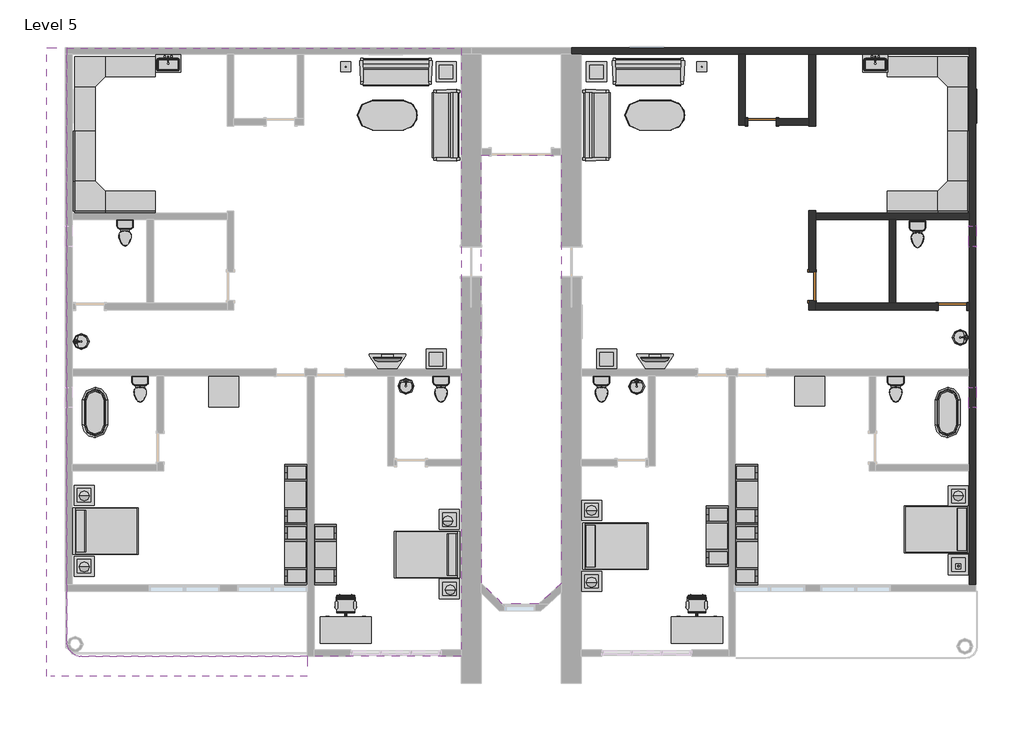
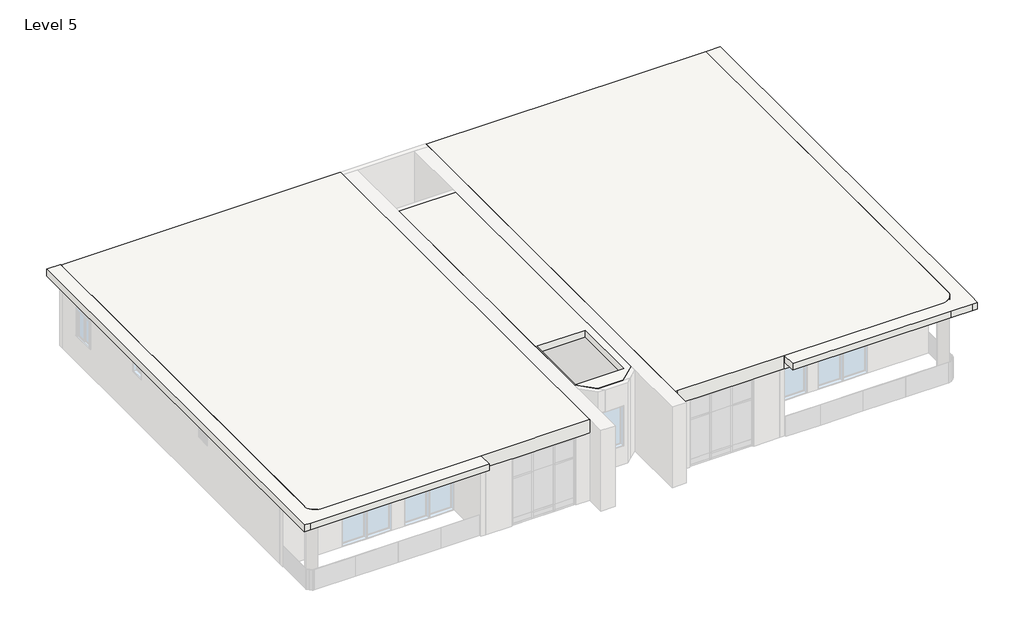
# One storey, part 3 of 3: 42 furniture elements, 14 flow terminals, 10 light fixtures, 9 walls, 3 doors, 3 slabs, 3 windows.
"""IFC4 building model written with IfcOpenShell, lengths in millimetres."""

from ifc_helpers import new_model, si_unit, point, frame, frame_2d, origin, place, context, project, spatial, polyline, circle_curve, trimmed, segment, composite_curve, outline, extrude, faceted_brep, transform, mapped, element, save
from components import door_2703ae13, door_10fd3a06, flow_terminal_38af2918, flow_terminal_d49f872f, toilet_domestic_3d_toilet_domestic_3d_f7549cf7, toilet_domestic_3d_toilet_domestic_3d_183bbd19, flow_terminal_b374fae2, furniture_07436f11, furniture_096e7f55, chair_task_arms_chair_task_arms_fa5a08ef, furniture_072f6425, furniture_cf0b6580, furniture_aff9b2fb, furniture_56245f3a, tv_stand_tv_stand_6ce107e5, furniture_b5c51a22, furniture_2c34a4f9, furniture_4d44e21c, furniture_45e3acac, light_fixture_100w_120v_8564026f, table_lamp_hemispheric_60w_120v_02721d88, window_0038ecf3, window_54100e87

model = new_model("IFC4")

# Units and contexts
model_context = context("Model", 3, world=origin())
ifc_project = project(units=[si_unit("LENGTHUNIT", "METRE", prefix="MILLI")], contexts=[model_context])

# Site, building, storey
site = spatial("IfcSite", under=ifc_project)
building = spatial("IfcBuilding", under=site)
storey = spatial("IfcBuildingStorey", under=building, Name="Level 5", Elevation=14630.4)

# Doors
placement = place(None, origin())
door_shape = door_2703ae13(model_context)
element("IfcDoor", 1, ObjectType="Door-Single-Panel.0001 : 34\" x 80\"", at=placement, inside=storey, context=model_context, shape_type="MappedRepresentation", body=[
    mapped(door_shape, transform((2522.0012296, 9464.0758558, 14630.4), x_axis=(-1.0, 0.0, 0.0), y_axis=(0.0, -1.0, 0.0), z_axis=(0.0, 0.0, 1.0))),
])
door_2_shape = door_10fd3a06(model_context)
element("IfcDoor", 2, ObjectType="Door-Single-Panel.0001 : 34\" x 80\"", at=placement, inside=storey, context=model_context, shape_type="MappedRepresentation", body=[
    mapped(door_2_shape, transform((8313.2012296, 3850.6758558, 14630.4), x_axis=(1.0, 0.0, 0.0), y_axis=(0.0, 1.0, 0.0), z_axis=(0.0, 0.0, 1.0))),
])
element("IfcDoor", 3, ObjectType="Door-Single-Panel.0001 : 34\" x 80\"", at=placement, inside=storey, context=model_context, shape_type="MappedRepresentation", body=[
    mapped(door_2_shape, transform((4046.0012296, 4460.2758558, 14630.4), x_axis=(0.0, -1.0, 0.0), y_axis=(1.0, 0.0, 0.0), z_axis=(0.0, 0.0, 1.0))),
])

# Flow terminals
flow_terminal_shape = flow_terminal_38af2918(model_context)
element("IfcFlowTerminal", 4, ObjectType="Sink Kitchen-Single : 30\" x 21\"", at=placement, inside=storey, context=model_context, shape_type="MappedRepresentation", body=[
    mapped(flow_terminal_shape, transform((-15540.388011, 11239.7304546, 14630.4), x_axis=(1.0, 0.0, 0.0), y_axis=(0.0, 1.0, 0.0), z_axis=(0.0, 0.0, 1.0))),
])
element("IfcFlowTerminal", 5, ObjectType="Sink Kitchen-Single : 30\" x 21\"", at=placement, inside=storey, context=model_context, shape_type="MappedRepresentation", body=[
    mapped(flow_terminal_shape, transform((5948.011989, 11239.7304546, 14630.4), x_axis=(1.0, 0.0, 0.0), y_axis=(0.0, 1.0, 0.0), z_axis=(0.0, 0.0, 1.0))),
])
flow_terminal_2_shape = flow_terminal_d49f872f(model_context)
element("IfcFlowTerminal", 6, ObjectType="Sink Vanity-Round : 19\" x 19\"", at=placement, inside=storey, context=model_context, shape_type="MappedRepresentation", body=[
    mapped(flow_terminal_2_shape, transform((-18084.6070794, 2687.2241152, 14630.4), x_axis=(0.0, 1.0, 0.0), y_axis=(-1.0, 0.0, 0.0), z_axis=(0.0, 0.0, 1.0))),
])
element("IfcFlowTerminal", 7, ObjectType="Sink Vanity-Round : 19\" x 19\"", at=placement, inside=storey, context=model_context, shape_type="MappedRepresentation", body=[
    mapped(flow_terminal_2_shape, transform((8462.2249463, 3007.5275963, 14630.4), x_axis=(0.0, -1.0, 0.0), y_axis=(1.0, 0.0, 0.0), z_axis=(0.0, 0.0, 1.0))),
])
element("IfcFlowTerminal", 8, ObjectType="Sink Vanity-Round : 19\" x 19\"", at=placement, inside=storey, context=model_context, shape_type="MappedRepresentation", body=[
    mapped(flow_terminal_2_shape, transform((-8395.050511, 1341.8921141, 14630.4), x_axis=(1.0, 0.0, 0.0), y_axis=(0.0, 1.0, 0.0), z_axis=(0.0, 0.0, 1.0))),
])
element("IfcFlowTerminal", 9, ObjectType="Sink Vanity-Round : 19\" x 19\"", at=placement, inside=storey, context=model_context, shape_type="MappedRepresentation", body=[
    mapped(flow_terminal_2_shape, transform((-1384.650511, 1331.0855344, 14630.4), x_axis=(1.0, 0.0, 0.0), y_axis=(0.0, 1.0, 0.0), z_axis=(0.0, 0.0, 1.0))),
])
toilet_domestic_3d_toilet_domestic_3d_shape = toilet_domestic_3d_toilet_domestic_3d_f7549cf7(model_context)
toilet_domestic_3d_toilet_domestic_3d_2_shape = toilet_domestic_3d_toilet_domestic_3d_183bbd19(model_context)
element("IfcFlowTerminal", 10, ObjectType="Toilet-Domestic-3D : Toilet-Domestic-3D", at=placement, inside=storey, context=model_context, shape_type="MappedRepresentation", body=[
    mapped(toilet_domestic_3d_toilet_domestic_3d_shape, transform((6586.0012296, 1247.7798284, 14630.4), x_axis=(1.0, 0.0, 0.0), y_axis=(0.0, 1.0, 0.0), z_axis=(0.0, 0.0, 1.0))),
    mapped(toilet_domestic_3d_toilet_domestic_3d_2_shape, transform((6586.0012296, 1247.7798284, 14630.4), x_axis=(1.0, 0.0, 0.0), y_axis=(0.0, 1.0, 0.0), z_axis=(0.0, 0.0, 1.0))),
])
element("IfcFlowTerminal", 11, ObjectType="Toilet-Domestic-3D : Toilet-Domestic-3D", at=placement, inside=storey, context=model_context, shape_type="MappedRepresentation", body=[
    mapped(toilet_domestic_3d_toilet_domestic_3d_shape, transform((-2354.7987704, 1247.7798284, 14630.4), x_axis=(1.0, 0.0, 0.0), y_axis=(0.0, 1.0, 0.0), z_axis=(0.0, 0.0, 1.0))),
    mapped(toilet_domestic_3d_toilet_domestic_3d_2_shape, transform((-2354.7987704, 1247.7798284, 14630.4), x_axis=(1.0, 0.0, 0.0), y_axis=(0.0, 1.0, 0.0), z_axis=(0.0, 0.0, 1.0))),
])
element("IfcFlowTerminal", 12, ObjectType="Toilet-Domestic-3D : Toilet-Domestic-3D", at=placement, inside=storey, context=model_context, shape_type="MappedRepresentation", body=[
    mapped(toilet_domestic_3d_toilet_domestic_3d_shape, transform((-16375.5987704, 1247.7798284, 14630.4), x_axis=(1.0, 0.0, 0.0), y_axis=(0.0, 1.0, 0.0), z_axis=(0.0, 0.0, 1.0))),
    mapped(toilet_domestic_3d_toilet_domestic_3d_2_shape, transform((-16375.5987704, 1247.7798284, 14630.4), x_axis=(1.0, 0.0, 0.0), y_axis=(0.0, 1.0, 0.0), z_axis=(0.0, 0.0, 1.0))),
])
element("IfcFlowTerminal", 13, ObjectType="Toilet-Domestic-3D : Toilet-Domestic-3D", at=placement, inside=storey, context=model_context, shape_type="MappedRepresentation", body=[
    mapped(toilet_domestic_3d_toilet_domestic_3d_shape, transform((-16832.7987704, 5997.5798284, 14630.4), x_axis=(1.0, 0.0, 0.0), y_axis=(0.0, 1.0, 0.0), z_axis=(0.0, 0.0, 1.0))),
    mapped(toilet_domestic_3d_toilet_domestic_3d_2_shape, transform((-16832.7987704, 5997.5798284, 14630.4), x_axis=(1.0, 0.0, 0.0), y_axis=(0.0, 1.0, 0.0), z_axis=(0.0, 0.0, 1.0))),
])
element("IfcFlowTerminal", 14, ObjectType="Toilet-Domestic-3D : Toilet-Domestic-3D", at=placement, inside=storey, context=model_context, shape_type="MappedRepresentation", body=[
    mapped(toilet_domestic_3d_toilet_domestic_3d_shape, transform((7246.4012296, 5946.7798284, 14630.4), x_axis=(1.0, 0.0, 0.0), y_axis=(0.0, 1.0, 0.0), z_axis=(0.0, 0.0, 1.0))),
    mapped(toilet_domestic_3d_toilet_domestic_3d_2_shape, transform((7246.4012296, 5946.7798284, 14630.4), x_axis=(1.0, 0.0, 0.0), y_axis=(0.0, 1.0, 0.0), z_axis=(0.0, 0.0, 1.0))),
])
element("IfcFlowTerminal", 15, ObjectType="Toilet-Domestic-3D : Toilet-Domestic-3D", at=placement, inside=storey, context=model_context, shape_type="MappedRepresentation", body=[
    mapped(toilet_domestic_3d_toilet_domestic_3d_shape, transform((-7231.5987704, 1247.7798284, 14630.4), x_axis=(1.0, 0.0, 0.0), y_axis=(0.0, 1.0, 0.0), z_axis=(0.0, 0.0, 1.0))),
    mapped(toilet_domestic_3d_toilet_domestic_3d_2_shape, transform((-7231.5987704, 1247.7798284, 14630.4), x_axis=(1.0, 0.0, 0.0), y_axis=(0.0, 1.0, 0.0), z_axis=(0.0, 0.0, 1.0))),
])
flow_terminal_3_shape = flow_terminal_b374fae2(model_context)
element("IfcFlowTerminal", 16, ObjectType="Tub-Free Standing-3D : 30\" x 60\"", at=placement, inside=storey, context=model_context, shape_type="MappedRepresentation", body=[
    mapped(flow_terminal_3_shape, transform((-17747.1987704, 624.8758558, 14630.4), x_axis=(1.0, 0.0, 0.0), y_axis=(0.0, 1.0, 0.0), z_axis=(0.0, 0.0, 1.0))),
])
element("IfcFlowTerminal", 17, ObjectType="Tub-Free Standing-3D : 30\" x 60\"", at=placement, inside=storey, context=model_context, shape_type="MappedRepresentation", body=[
    mapped(flow_terminal_3_shape, transform((8160.8012296, 624.8758558, 14630.4), x_axis=(1.0, 0.0, 0.0), y_axis=(0.0, 1.0, 0.0), z_axis=(0.0, 0.0, 1.0))),
])

# Furniture
furniture_shape = furniture_07436f11(model_context)
element("IfcFurniture", 18, ObjectType="96\" x 96\"", at=placement, inside=storey, context=model_context, shape_type="MappedRepresentation", body=[
    mapped(furniture_shape, transform((-18275.8670182, 11991.0988634, 14630.4), x_axis=(1.0, 0.0, 0.0), y_axis=(0.0, 1.0, 0.0), z_axis=(0.0, 0.0, 1.0))),
])
element("IfcFurniture", 19, ObjectType="96\" x 96\"", at=placement, inside=storey, context=model_context, shape_type="MappedRepresentation", body=[
    mapped(furniture_shape, transform((9316.2242372, 11364.3441035, 14630.4), x_axis=(0.0, -1.0, 0.0), y_axis=(1.0, 0.0, 0.0), z_axis=(0.0, 0.0, 1.0))),
])
furniture_2_shape = furniture_096e7f55(model_context)
element("IfcFurniture", 20, ObjectType="Bed-Shaker : Double 56\" x 78\"", at=placement, inside=storey, context=model_context, shape_type="MappedRepresentation", body=[
    mapped(furniture_2_shape, transform((-18407.5987704, -2962.8741442, 14630.4), x_axis=(0.0, 1.0, 0.0), y_axis=(-1.0, 0.0, 0.0), z_axis=(0.0, 0.0, 1.0))),
])
element("IfcFurniture", 21, ObjectType="Bed-Shaker : Double 56\" x 78\"", at=placement, inside=storey, context=model_context, shape_type="MappedRepresentation", body=[
    mapped(furniture_2_shape, transform((-6672.7987704, -3712.1741442, 14630.4), x_axis=(0.0, -1.0, 0.0), y_axis=(1.0, 0.0, 0.0), z_axis=(0.0, 0.0, 1.0))),
])
element("IfcFurniture", 22, ObjectType="Bed-Shaker : Double 56\" x 78\"", at=placement, inside=storey, context=model_context, shape_type="MappedRepresentation", body=[
    mapped(furniture_2_shape, transform((-2913.5987704, -3420.0741442, 14630.4), x_axis=(0.0, 1.0, 0.0), y_axis=(-1.0, 0.0, 0.0), z_axis=(0.0, 0.0, 1.0))),
])
element("IfcFurniture", 23, ObjectType="Bed-Shaker : Double 56\" x 78\"", at=placement, inside=storey, context=model_context, shape_type="MappedRepresentation", body=[
    mapped(furniture_2_shape, transform((8821.2012296, -2950.1741442, 14630.4), x_axis=(0.0, -1.0, 0.0), y_axis=(1.0, 0.0, 0.0), z_axis=(0.0, 0.0, 1.0))),
])
chair_task_arms_chair_task_arms_shape = chair_task_arms_chair_task_arms_fa5a08ef(model_context)
element("IfcFurniture", 24, ObjectType="Chair-Task Arms : Chair-Task Arms", at=placement, inside=storey, context=model_context, shape_type="MappedRepresentation", body=[
    mapped(chair_task_arms_chair_task_arms_shape, transform((681.7920493, -5184.3566833, 14630.4), x_axis=(-1.0, 0.0, 0.0), y_axis=(0.0, -1.0, 0.0), z_axis=(0.0, 0.0, 1.0))),
])
element("IfcFurniture", 25, ObjectType="Chair-Task Arms : Chair-Task Arms", at=placement, inside=storey, context=model_context, shape_type="MappedRepresentation", body=[
    mapped(chair_task_arms_chair_task_arms_shape, transform((-9986.2079507, -5184.3566833, 14630.4), x_axis=(-1.0, 0.0, 0.0), y_axis=(0.0, -1.0, 0.0), z_axis=(0.0, 0.0, 1.0))),
])
furniture_3_shape = furniture_072f6425(model_context)
element("IfcFurniture", 26, ObjectType="Desk : 60\" x 30\"", at=placement, inside=storey, context=model_context, shape_type="MappedRepresentation", body=[
    mapped(furniture_3_shape, transform((-10889.1987704, -6371.702585, 14630.4), x_axis=(1.0, 0.0, 0.0), y_axis=(0.0, 1.0, 0.0), z_axis=(0.0, 0.0, 1.0))),
])
element("IfcFurniture", 27, ObjectType="Desk : 60\" x 30\"", at=placement, inside=storey, context=model_context, shape_type="MappedRepresentation", body=[
    mapped(furniture_3_shape, transform((-221.1987704, -6371.702585, 14630.4), x_axis=(1.0, 0.0, 0.0), y_axis=(0.0, 1.0, 0.0), z_axis=(0.0, 0.0, 1.0))),
])
furniture_4_shape = furniture_cf0b6580(model_context)
element("IfcFurniture", 28, ObjectType="Entertainment Center : 72\" x 72\" x 24\"", at=placement, inside=storey, context=model_context, shape_type="MappedRepresentation", body=[
    mapped(furniture_4_shape, transform((1607.6012296, -3134.3241442, 14630.4), x_axis=(0.0, -1.0, 0.0), y_axis=(1.0, 0.0, 0.0), z_axis=(0.0, 0.0, 1.0))),
])
element("IfcFurniture", 29, ObjectType="Entertainment Center : 72\" x 72\" x 24\"", at=placement, inside=storey, context=model_context, shape_type="MappedRepresentation", body=[
    mapped(furniture_4_shape, transform((1607.6012296, -3693.1241442, 14630.4), x_axis=(0.0, 1.0, 0.0), y_axis=(-1.0, 0.0, 0.0), z_axis=(0.0, 0.0, 1.0))),
])
element("IfcFurniture", 30, ObjectType="Entertainment Center : 72\" x 72\" x 24\"", at=placement, inside=storey, context=model_context, shape_type="MappedRepresentation", body=[
    mapped(furniture_4_shape, transform((1607.6012296, -1864.3241442, 14630.4), x_axis=(0.0, 1.0, 0.0), y_axis=(-1.0, 0.0, 0.0), z_axis=(0.0, 0.0, 1.0))),
])
element("IfcFurniture", 31, ObjectType="Entertainment Center : 72\" x 72\" x 24\"", at=placement, inside=storey, context=model_context, shape_type="MappedRepresentation", body=[
    mapped(furniture_4_shape, transform((-11193.9987704, -3693.1241442, 14630.4), x_axis=(0.0, -1.0, 0.0), y_axis=(1.0, 0.0, 0.0), z_axis=(0.0, 0.0, 1.0))),
])
element("IfcFurniture", 32, ObjectType="Entertainment Center : 72\" x 72\" x 24\"", at=placement, inside=storey, context=model_context, shape_type="MappedRepresentation", body=[
    mapped(furniture_4_shape, transform((-11193.9987704, -1864.3241442, 14630.4), x_axis=(0.0, -1.0, 0.0), y_axis=(1.0, 0.0, 0.0), z_axis=(0.0, 0.0, 1.0))),
])
element("IfcFurniture", 33, ObjectType="Entertainment Center : 72\" x 72\" x 24\"", at=placement, inside=storey, context=model_context, shape_type="MappedRepresentation", body=[
    mapped(furniture_4_shape, transform((-11193.9987704, -3693.1241442, 14630.4), x_axis=(0.0, 1.0, 0.0), y_axis=(-1.0, 0.0, 0.0), z_axis=(0.0, 0.0, 1.0))),
])
furniture_5_shape = furniture_aff9b2fb(model_context)
element("IfcFurniture", 34, ObjectType="Sofa-Pensi : 84\"", at=placement, inside=storey, context=model_context, shape_type="MappedRepresentation", body=[
    mapped(furniture_5_shape, transform((-8881.8050204, 10710.9660197, 14630.4), x_axis=(1.0, 0.0, 0.0), y_axis=(0.0, 1.0, 0.0), z_axis=(0.0, 0.0, 1.0))),
])
element("IfcFurniture", 35, ObjectType="Sofa-Pensi : 84\"", at=placement, inside=storey, context=model_context, shape_type="MappedRepresentation", body=[
    mapped(furniture_5_shape, transform((-7356.3086065, 9641.0821058, 14630.4), x_axis=(0.0, -1.0, 0.0), y_axis=(1.0, 0.0, 0.0), z_axis=(0.0, 0.0, 1.0))),
])
element("IfcFurniture", 36, ObjectType="Sofa-Pensi : 84\"", at=placement, inside=storey, context=model_context, shape_type="MappedRepresentation", body=[
    mapped(furniture_5_shape, transform((-2230.0889343, 9083.8696058, 14630.4), x_axis=(0.0, 1.0, 0.0), y_axis=(-1.0, 0.0, 0.0), z_axis=(0.0, 0.0, 1.0))),
])
element("IfcFurniture", 37, ObjectType="Sofa-Pensi : 84\"", at=placement, inside=storey, context=model_context, shape_type="MappedRepresentation", body=[
    mapped(furniture_5_shape, transform((-1211.0050204, 10710.9660197, 14630.4), x_axis=(1.0, 0.0, 0.0), y_axis=(0.0, 1.0, 0.0), z_axis=(0.0, 0.0, 1.0))),
])
furniture_6_shape = furniture_56245f3a(model_context)
element("IfcFurniture", 38, ObjectType="TV - Flat Screen : 32\"", at=placement, inside=storey, context=model_context, shape_type="MappedRepresentation", body=[
    mapped(furniture_6_shape, transform((-8861.1432846, 2232.8144794, 15544.8), x_axis=(-1.0, 0.0, 0.0), y_axis=(0.0, -1.0, 0.0), z_axis=(0.0, 0.0, 1.0))),
])
element("IfcFurniture", 39, ObjectType="TV - Flat Screen : 32\"", at=placement, inside=storey, context=model_context, shape_type="MappedRepresentation", body=[
    mapped(furniture_6_shape, transform((-733.1432846, 2232.8144794, 15544.8), x_axis=(-1.0, 0.0, 0.0), y_axis=(0.0, -1.0, 0.0), z_axis=(0.0, 0.0, 1.0))),
])
tv_stand_tv_stand_shape = tv_stand_tv_stand_6ce107e5(model_context)
element("IfcFurniture", 40, ObjectType="TV Stand : TV Stand", at=placement, inside=storey, context=model_context, shape_type="MappedRepresentation", body=[
    mapped(tv_stand_tv_stand_shape, transform((-8732.0107683, 1945.6758558, 14630.4), x_axis=(-1.0, 0.0, 0.0), y_axis=(0.0, -1.0, 0.0), z_axis=(0.0, 0.0, 1.0))),
])
element("IfcFurniture", 41, ObjectType="TV Stand : TV Stand", at=placement, inside=storey, context=model_context, shape_type="MappedRepresentation", body=[
    mapped(tv_stand_tv_stand_shape, transform((-604.0107683, 1945.6758558, 14630.4), x_axis=(-1.0, 0.0, 0.0), y_axis=(0.0, -1.0, 0.0), z_axis=(0.0, 0.0, 1.0))),
])
furniture_7_shape = furniture_b5c51a22(model_context)
element("IfcFurniture", 42, ObjectType="Table-Coffee : 24\" x 24\" x 24\"", at=placement, inside=storey, context=model_context, shape_type="MappedRepresentation", body=[
    mapped(furniture_7_shape, transform((-7097.4645371, 10892.864778, 14630.4), x_axis=(1.0, 0.0, 0.0), y_axis=(0.0, 1.0, 0.0), z_axis=(0.0, 0.0, 1.0))),
])
element("IfcFurniture", 43, ObjectType="Table-Coffee : 24\" x 24\" x 24\"", at=placement, inside=storey, context=model_context, shape_type="MappedRepresentation", body=[
    mapped(furniture_7_shape, transform((-2525.4645371, 10892.864778, 14630.4), x_axis=(1.0, 0.0, 0.0), y_axis=(0.0, 1.0, 0.0), z_axis=(0.0, 0.0, 1.0))),
])
element("IfcFurniture", 44, ObjectType="Table-Coffee : 24\" x 24\" x 24\"", at=placement, inside=storey, context=model_context, shape_type="MappedRepresentation", body=[
    mapped(furniture_7_shape, transform((-7402.2645371, 2155.264778, 14630.4), x_axis=(1.0, 0.0, 0.0), y_axis=(0.0, 1.0, 0.0), z_axis=(0.0, 0.0, 1.0))),
])
element("IfcFurniture", 45, ObjectType="Table-Coffee : 24\" x 24\" x 24\"", at=placement, inside=storey, context=model_context, shape_type="MappedRepresentation", body=[
    mapped(furniture_7_shape, transform((-2220.6645371, 2155.264778, 14630.4), x_axis=(1.0, 0.0, 0.0), y_axis=(0.0, 1.0, 0.0), z_axis=(0.0, 0.0, 1.0))),
])
element("IfcFurniture", 46, ObjectType="Table-Coffee : 24\" x 24\" x 24\"", at=placement, inside=storey, context=model_context, shape_type="MappedRepresentation", body=[
    mapped(furniture_7_shape, transform((-2677.8645371, -4601.135222, 14630.4), x_axis=(1.0, 0.0, 0.0), y_axis=(0.0, 1.0, 0.0), z_axis=(0.0, 0.0, 1.0))),
])
element("IfcFurniture", 47, ObjectType="Table-Coffee : 24\" x 24\" x 24\"", at=placement, inside=storey, context=model_context, shape_type="MappedRepresentation", body=[
    mapped(furniture_7_shape, transform((-18095.6645371, -4143.935222, 14630.4), x_axis=(1.0, 0.0, 0.0), y_axis=(0.0, 1.0, 0.0), z_axis=(0.0, 0.0, 1.0))),
])
element("IfcFurniture", 48, ObjectType="Table-Coffee : 24\" x 24\" x 24\"", at=placement, inside=storey, context=model_context, shape_type="MappedRepresentation", body=[
    mapped(furniture_7_shape, transform((-18095.6645371, -1984.935222, 14630.4), x_axis=(1.0, 0.0, 0.0), y_axis=(0.0, 1.0, 0.0), z_axis=(0.0, 0.0, 1.0))),
])
element("IfcFurniture", 49, ObjectType="Table-Coffee : 24\" x 24\" x 24\"", at=placement, inside=storey, context=model_context, shape_type="MappedRepresentation", body=[
    mapped(furniture_7_shape, transform((-2677.8645371, -2442.135222, 14630.4), x_axis=(1.0, 0.0, 0.0), y_axis=(0.0, 1.0, 0.0), z_axis=(0.0, 0.0, 1.0))),
])
element("IfcFurniture", 50, ObjectType="Table-Coffee : 24\" x 24\" x 24\"", at=placement, inside=storey, context=model_context, shape_type="MappedRepresentation", body=[
    mapped(furniture_7_shape, transform((8472.7354629, -4093.135222, 14630.4), x_axis=(1.0, 0.0, 0.0), y_axis=(0.0, 1.0, 0.0), z_axis=(0.0, 0.0, 1.0))),
])
element("IfcFurniture", 51, ObjectType="Table-Coffee : 24\" x 24\" x 24\"", at=placement, inside=storey, context=model_context, shape_type="MappedRepresentation", body=[
    mapped(furniture_7_shape, transform((8472.7354629, -2010.335222, 14630.4), x_axis=(1.0, 0.0, 0.0), y_axis=(0.0, 1.0, 0.0), z_axis=(0.0, 0.0, 1.0))),
])
element("IfcFurniture", 52, ObjectType="Table-Coffee : 24\" x 24\" x 24\"", at=placement, inside=storey, context=model_context, shape_type="MappedRepresentation", body=[
    mapped(furniture_7_shape, transform((-6995.8645371, -4832.0414601, 14630.4), x_axis=(1.0, 0.0, 0.0), y_axis=(0.0, 1.0, 0.0), z_axis=(0.0, 0.0, 1.0))),
])
element("IfcFurniture", 53, ObjectType="Table-Coffee : 24\" x 24\" x 24\"", at=placement, inside=storey, context=model_context, shape_type="MappedRepresentation", body=[
    mapped(furniture_7_shape, transform((-6995.8645371, -2723.8414601, 14630.4), x_axis=(1.0, 0.0, 0.0), y_axis=(0.0, 1.0, 0.0), z_axis=(0.0, 0.0, 1.0))),
])
furniture_8_shape = furniture_2c34a4f9(model_context)
element("IfcFurniture", 54, ObjectType="Table-Dining Oval : 36\" x 72\"", at=placement, inside=storey, context=model_context, shape_type="MappedRepresentation", body=[
    mapped(furniture_8_shape, transform((-8455.3790983, 10025.3742164, 14630.4), x_axis=(1.0, 0.0, 0.0), y_axis=(0.0, 1.0, 0.0), z_axis=(0.0, 0.0, 1.0))),
])
element("IfcFurniture", 55, ObjectType="Table-Dining Oval : 36\" x 72\"", at=placement, inside=storey, context=model_context, shape_type="MappedRepresentation", body=[
    mapped(furniture_8_shape, transform((-327.3790983, 10025.3742164, 14630.4), x_axis=(1.0, 0.0, 0.0), y_axis=(0.0, 1.0, 0.0), z_axis=(0.0, 0.0, 1.0))),
])
furniture_9_shape = furniture_4d44e21c(model_context)
element("IfcFurniture", 56, ObjectType="Table-Rectangular : 36\" x 36\"", at=placement, inside=storey, context=model_context, shape_type="MappedRepresentation", body=[
    mapped(furniture_9_shape, transform((-13835.5987704, 1259.8758558, 14630.4), x_axis=(1.0, 0.0, 0.0), y_axis=(0.0, 1.0, 0.0), z_axis=(0.0, 0.0, 1.0))),
])
element("IfcFurniture", 57, ObjectType="Table-Rectangular : 36\" x 36\"", at=placement, inside=storey, context=model_context, shape_type="MappedRepresentation", body=[
    mapped(furniture_9_shape, transform((3969.8012296, 1285.2758558, 14630.4), x_axis=(1.0, 0.0, 0.0), y_axis=(0.0, 1.0, 0.0), z_axis=(0.0, 0.0, 1.0))),
])
furniture_10_shape = furniture_45e3acac(model_context)
element("IfcFurniture", 58, ObjectType="Work Station Cubicle : 96\" x 96\"", at=placement, inside=storey, context=model_context, shape_type="MappedRepresentation", body=[
    mapped(furniture_10_shape, transform((-18902.621778, 6827.207608, 14630.4), x_axis=(0.0, 1.0, 0.0), y_axis=(-1.0, 0.0, 0.0), z_axis=(0.0, 0.0, 1.0))),
])
element("IfcFurniture", 59, ObjectType="Work Station Cubicle : 96\" x 96\"", at=placement, inside=storey, context=model_context, shape_type="MappedRepresentation", body=[
    mapped(furniture_10_shape, transform((8689.4694774, 6200.4528481, 14630.4), x_axis=(-1.0, 0.0, 0.0), y_axis=(0.0, -1.0, 0.0), z_axis=(0.0, 0.0, 1.0))),
])

# Light fixtures
light_fixture_100w_120v_shape = light_fixture_100w_120v_8564026f(model_context)
element("IfcLightFixture", 60, ObjectType="100W - 120V", at=placement, inside=storey, context=model_context, shape_type="MappedRepresentation", body=[
    mapped(light_fixture_100w_120v_shape, transform((-10127.1987704, 11140.4758558, 14630.4), x_axis=(1.0, 0.0, 0.0), y_axis=(0.0, 1.0, 0.0), z_axis=(0.0, 0.0, 1.0))),
])
element("IfcLightFixture", 61, ObjectType="100W - 120V", at=placement, inside=storey, context=model_context, shape_type="MappedRepresentation", body=[
    mapped(light_fixture_100w_120v_shape, transform((693.2012296, 11140.4758558, 14630.4), x_axis=(1.0, 0.0, 0.0), y_axis=(0.0, 1.0, 0.0), z_axis=(0.0, 0.0, 1.0))),
])
table_lamp_hemispheric_60w_120v_shape = table_lamp_hemispheric_60w_120v_02721d88(model_context)
element("IfcLightFixture", 62, ObjectType="Table Lamp - Hemispheric : 60W - 120V", at=placement, inside=storey, context=model_context, shape_type="MappedRepresentation", body=[
    mapped(table_lamp_hemispheric_60w_120v_shape, transform((-18077.3987704, -1915.1241442, 15240.0), x_axis=(1.0, 0.0, 0.0), y_axis=(0.0, 1.0, 0.0), z_axis=(0.0, 0.0, 1.0))),
])
element("IfcLightFixture", 63, ObjectType="Table Lamp - Hemispheric : 60W - 120V", at=placement, inside=storey, context=model_context, shape_type="MappedRepresentation", body=[
    mapped(table_lamp_hemispheric_60w_120v_shape, transform((-7028.3987704, -2666.7303823, 15240.0), x_axis=(1.0, 0.0, 0.0), y_axis=(0.0, 1.0, 0.0), z_axis=(0.0, 0.0, 1.0))),
])
element("IfcLightFixture", 64, ObjectType="Table Lamp - Hemispheric : 60W - 120V", at=placement, inside=storey, context=model_context, shape_type="MappedRepresentation", body=[
    mapped(table_lamp_hemispheric_60w_120v_shape, transform((-2659.5987704, -2346.9241442, 15240.0), x_axis=(1.0, 0.0, 0.0), y_axis=(0.0, 1.0, 0.0), z_axis=(0.0, 0.0, 1.0))),
])
element("IfcLightFixture", 65, ObjectType="Table Lamp - Hemispheric : 60W - 120V", at=placement, inside=storey, context=model_context, shape_type="MappedRepresentation", body=[
    mapped(table_lamp_hemispheric_60w_120v_shape, transform((8491.0012296, -4048.7241442, 15544.8), x_axis=(1.0, 0.0, 0.0), y_axis=(0.0, 1.0, 0.0), z_axis=(0.0, 0.0, 1.0))),
])
element("IfcLightFixture", 66, ObjectType="Table Lamp - Hemispheric : 60W - 120V", at=placement, inside=storey, context=model_context, shape_type="MappedRepresentation", body=[
    mapped(table_lamp_hemispheric_60w_120v_shape, transform((8491.0012296, -1915.1241442, 15240.0), x_axis=(1.0, 0.0, 0.0), y_axis=(0.0, 1.0, 0.0), z_axis=(0.0, 0.0, 1.0))),
])
element("IfcLightFixture", 67, ObjectType="Table Lamp - Hemispheric : 60W - 120V", at=placement, inside=storey, context=model_context, shape_type="MappedRepresentation", body=[
    mapped(table_lamp_hemispheric_60w_120v_shape, transform((-2659.5987704, -4531.3241442, 15240.0), x_axis=(1.0, 0.0, 0.0), y_axis=(0.0, 1.0, 0.0), z_axis=(0.0, 0.0, 1.0))),
])
element("IfcLightFixture", 68, ObjectType="Table Lamp - Hemispheric : 60W - 120V", at=placement, inside=storey, context=model_context, shape_type="MappedRepresentation", body=[
    mapped(table_lamp_hemispheric_60w_120v_shape, transform((-6952.1987704, -4762.2303823, 15240.0), x_axis=(1.0, 0.0, 0.0), y_axis=(0.0, 1.0, 0.0), z_axis=(0.0, 0.0, 1.0))),
])
element("IfcLightFixture", 69, ObjectType="Table Lamp - Hemispheric : 60W - 120V", at=placement, inside=storey, context=model_context, shape_type="MappedRepresentation", body=[
    mapped(table_lamp_hemispheric_60w_120v_shape, transform((-18077.3987704, -4074.1241442, 15240.0), x_axis=(1.0, 0.0, 0.0), y_axis=(0.0, 1.0, 0.0), z_axis=(0.0, 0.0, 1.0))),
])

# Slabs
element("IfcSlab", 70, ObjectType="Generic - 12\" cream", at=placement, inside=storey, context=model_context, shape_type="SweptSolid", body=[
    extrude(outline(composite_curve([segment(polyline([(-6621.9987704, 11699.2758558), (-6621.9987704, -6791.9241442), (-11295.5987704, -6791.9241442), (-18153.5987704, -6791.9241442)]), True, "CONTINUOUS"), segment(trimmed(circle_curve(frame_2d((-18153.5987704, -6334.7241442)), 457.2), [point((-18153.5987704, -6791.9241442))], [point((-18610.7987704, -6334.7241442))], False, "CARTESIAN"), True, "CONTINUOUS"), segment(polyline([(-18610.7987704, -6334.7241442), (-18610.7987704, 11699.2758558), (-6621.9987704, 11699.2758558)]), True, "CONTINUOUS")], self_intersect=False)), frame((0.0, 0.0, 17678.4), z_axis=(0.0, 0.0, 1.0), x_axis=(1.0, 0.0, 0.0)), (0.0, 0.0, 1.0), 609.6),
    extrude(outline(composite_curve([segment(trimmed(circle_curve(frame_2d((8511.8043381, -6277.3874522)), 514.536692), [point((9024.4012296, -6322.0241442))], [point((8511.8043381, -6791.9241442))], False, "CARTESIAN"), True, "CONTINUOUS"), segment(polyline([(8511.8043381, -6791.9241442), (1709.2012296, -6791.9241442), (-2862.7987704, -6791.9241442), (-2964.3987704, -6791.9241442), (-2964.3987704, 11699.2758558), (9024.4012296, 11699.2758558), (9024.4012296, -6322.0241442)]), True, "CONTINUOUS")], self_intersect=False)), frame((0.0, 0.0, 17678.4), z_axis=(0.0, 0.0, 1.0), x_axis=(1.0, 0.0, 0.0)), (0.0, 0.0, 1.0), 609.6),
])
element("IfcSlab", 71, ObjectType="Generic - 12\" white", at=placement, inside=storey, context=model_context, shape_type="SweptSolid", body=[
    extrude(outline(composite_curve([segment(polyline([(9634.0012296, 11699.2758558), (9634.0012296, -6931.6241442), (9634.0012296, -7401.5241442), (9430.8012296, -7401.5241442), (8511.8043381, -7401.5241442), (1709.2012296, -7401.5241442), (1709.2012296, -6791.9241442), (8511.8043381, -6791.9241442)]), True, "CONTINUOUS"), segment(trimmed(circle_curve(frame_2d((8511.8043381, -6277.3874522)), 514.536692), [point((8511.8043381, -6791.9241442))], [point((9024.4012296, -6322.0241442))], True, "CARTESIAN"), True, "CONTINUOUS"), segment(polyline([(9024.4012296, -6322.0241442), (9024.4012296, 11699.2758558), (9634.0012296, 11699.2758558)]), True, "CONTINUOUS")], self_intersect=False)), frame((0.0, 0.0, 17983.2), z_axis=(0.0, 0.0, 1.0), x_axis=(1.0, 0.0, 0.0)), (0.0, 0.0, 1.0), 304.8),
    extrude(outline(composite_curve([segment(polyline([(-18610.7987704, 11724.6758558), (-18610.7987704, -6334.7241442)]), True, "CONTINUOUS"), segment(trimmed(circle_curve(frame_2d((-18153.5987704, -6334.7241442)), 457.2), [point((-18610.7987704, -6334.7241442))], [point((-18153.5987704, -6791.9241442))], True, "CARTESIAN"), True, "CONTINUOUS"), segment(polyline([(-18153.5987704, -6791.9241442), (-11295.5987704, -6791.9241442), (-11295.5987704, -7401.5241442), (-18966.3987704, -7401.5241442), (-19220.3987704, -7401.5241442), (-19220.3987704, 11724.6758558), (-18610.7987704, 11724.6758558)]), True, "CONTINUOUS")], self_intersect=False)), frame((0.0, 0.0, 17983.2), z_axis=(0.0, 0.0, 1.0), x_axis=(1.0, 0.0, 0.0)), (0.0, 0.0, 1.0), 304.8),
])
element("IfcSlab", 72, ObjectType="Generic - 12\" white", at=placement, inside=storey, context=model_context, shape_type="SweptSolid", body=[
    extrude(outline(polyline([(-3573.9987704, 8448.0758558), (-3573.9987704, -1691.5549149), (-3573.9987704, -4572.9908503), (-4263.8661085, -5188.2185522), (-5369.3570449, -5188.2185522), (-5997.9749734, -4559.6006237), (-5997.9749734, -1691.5549149), (-6012.3987704, -1691.5549149), (-6012.3987704, 8448.0758558), (-3573.9987704, 8448.0758558)]), holes=[polyline([(-5940.8822214, -4561.7549149), (-3883.4822214, -4561.7549149), (-3883.4822214, -1691.5549149), (-5940.8822214, -1691.5549149), (-5940.8822214, -4561.7549149)])]), frame((0.0, 0.0, 17983.2), z_axis=(0.0, 0.0, 1.0), x_axis=(1.0, 0.0, 0.0)), (0.0, 0.0, 1.0), 304.8),
])

# Walls
element("IfcWall", 73, ObjectType="Generic - 8\" cream", at=placement, inside=storey, context=model_context, shape_type="Brep", body=[
    faceted_brep([(8821.2012296, 11724.6758558, 14630.4), (8821.2012296, 11521.4758558, 14630.4), (8821.2012296, 6695.4758558, 14630.4), (8821.2012296, 6492.2758558, 14630.4), (8821.2012296, 3952.2758558, 14630.4), (8821.2012296, 3749.0758558, 14630.4), (8821.2012296, 1945.6758558, 14630.4), (8821.2012296, 1742.4758558, 14630.4), (8821.2012296, -949.9241442, 14630.4), (8821.2012296, -1153.1241442, 14630.4), (8821.2012296, -4607.5241442, 14630.4), (8821.2012296, -4607.5241442, 17678.4), (8821.2012296, -1153.1241442, 17678.4), (8821.2012296, -949.9241442, 17678.4), (8821.2012296, 1742.4758558, 17678.4), (8821.2012296, 1945.6758558, 17678.4), (8821.2012296, 3749.0758558, 17678.4), (8821.2012296, 3952.2758558, 17678.4), (8821.2012296, 6492.2758558, 17678.4), (8821.2012296, 6695.4758558, 17678.4), (8821.2012296, 11521.4758558, 17678.4), (8821.2012296, 11724.6758558, 17678.4), (8821.2012296, 10403.8758558, 15849.6), (8821.2012296, 10403.8758558, 17068.8), (8821.2012296, 9489.4758558, 17068.8), (8821.2012296, 9489.4758558, 15849.6), (8821.2012296, 777.2758558, 17373.6), (8821.2012296, 777.2758558, 16764.0), (8821.2012296, 1386.8758558, 16764.0), (8821.2012296, 1386.8758558, 17373.6), (8821.2012296, 6289.0758558, 16764.0), (8821.2012296, 6289.0758558, 17373.6), (8821.2012296, 5679.4758558, 17373.6), (8821.2012296, 5679.4758558, 16764.0), (9024.4012296, -4607.5241442, 14630.4), (9024.4012296, 11724.6758558, 14630.4), (9024.4012296, 11724.6758558, 17678.4), (9024.4012296, -4607.5241442, 17678.4), (9024.4012296, 10403.8758558, 17068.8), (9024.4012296, 10403.8758558, 15849.6), (9024.4012296, 9489.4758558, 15849.6), (9024.4012296, 9489.4758558, 17068.8), (9024.4012296, 777.2758558, 16764.0), (9024.4012296, 777.2758558, 17373.6), (9024.4012296, 1386.8758558, 17373.6), (9024.4012296, 1386.8758558, 16764.0), (9024.4012296, 6289.0758558, 17373.6), (9024.4012296, 6289.0758558, 16764.0), (9024.4012296, 5679.4758558, 16764.0), (9024.4012296, 5679.4758558, 17373.6)], [[[0, 1, 2, 3, 4, 5, 6, 7, 8, 9, 10, 11, 12, 13, 14, 15, 16, 17, 18, 19, 20, 21], [22, 23, 24, 25], [26, 27, 28, 29], [30, 31, 32, 33]], [[34, 35, 36, 37], [38, 39, 40, 41], [42, 43, 44, 45], [46, 47, 48, 49]], [[10, 9, 8, 7, 6, 5, 4, 3, 2, 1, 0, 35, 34]], [[21, 20, 19, 18, 17, 16, 15, 14, 13, 12, 11, 37, 36]], [[0, 21, 36, 35]], [[11, 10, 34, 37]], [[39, 38, 23, 22]], [[40, 39, 22, 25]], [[41, 40, 25, 24]], [[38, 41, 24, 23]], [[26, 43, 42, 27]], [[27, 42, 45, 28]], [[28, 45, 44, 29]], [[43, 26, 29, 44]], [[46, 31, 30, 47]], [[47, 30, 33, 48]], [[48, 33, 32, 49]], [[31, 46, 49, 32]]]),
])
element("IfcWall", 74, ObjectType="Generic - 8\" cream", at=placement, inside=storey, context=model_context, shape_type="Brep", body=[
    faceted_brep([(3944.4012296, 11521.4758558, 14630.4), (3944.4012296, 9565.6758558, 14630.4), (3944.4012296, 9362.4758558, 14630.4), (3944.4012296, 9337.0758558, 14630.4), (3944.4012296, 9337.0758558, 17678.4), (3944.4012296, 9362.4758558, 17678.4), (3944.4012296, 9565.6758558, 17678.4), (3944.4012296, 11521.4758558, 17678.4), (4147.6012296, 11521.4758558, 14630.4), (4147.6012296, 11521.4758558, 17678.4), (4147.6012296, 9337.0758558, 17678.4), (4147.6012296, 9337.0758558, 14630.4)], [[[0, 1, 2, 3, 4, 5, 6, 7]], [[8, 9, 10, 11]], [[3, 2, 1, 0, 8, 11]], [[4, 3, 11, 10]], [[7, 6, 5, 4, 10, 9]], [[0, 7, 9, 8]]]),
])
element("IfcWall", 75, ObjectType="Generic - 8\" cream", at=placement, inside=storey, context=model_context, shape_type="Brep", body=[
    faceted_brep([(4147.6012296, 6492.2758558, 14630.4), (6382.8012296, 6492.2758558, 14630.4), (6586.0012296, 6492.2758558, 14630.4), (8821.2012296, 6492.2758558, 14630.4), (8821.2012296, 6492.2758558, 17678.4), (6586.0012296, 6492.2758558, 17678.4), (6382.8012296, 6492.2758558, 17678.4), (4147.6012296, 6492.2758558, 17678.4), (4147.6012296, 6695.4758558, 14630.4), (4147.6012296, 6695.4758558, 17678.4), (8821.2012296, 6695.4758558, 17678.4), (8821.2012296, 6695.4758558, 14630.4)], [[[0, 1, 2, 3, 4, 5, 6, 7]], [[8, 9, 10, 11]], [[3, 2, 1, 0, 8, 11]], [[7, 6, 5, 4, 10, 9]], [[0, 7, 9, 8]], [[4, 3, 11, 10]]]),
])
element("IfcWall", 76, ObjectType="Generic - 8\" cream", at=placement, inside=storey, context=model_context, shape_type="Brep", body=[
    faceted_brep([(8821.2012296, 3749.0758558, 17678.4), (4147.6012296, 3749.0758558, 17678.4), (4147.6012296, 3749.0758558, 14630.4), (7881.4012296, 3749.0758558, 14630.4), (7881.4012296, 3749.0758558, 16662.4), (8745.0012296, 3749.0758558, 16662.4), (8745.0012296, 3749.0758558, 14630.4), (8821.2012296, 3749.0758558, 14630.4), (4147.6012296, 3952.2758558, 17678.4), (6382.8012296, 3952.2758558, 17678.4), (6586.0012296, 3952.2758558, 17678.4), (8821.2012296, 3952.2758558, 17678.4), (8821.2012296, 3952.2758558, 14630.4), (8745.0012296, 3952.2758558, 14630.4), (8745.0012296, 3952.2758558, 16662.4), (7881.4012296, 3952.2758558, 16662.4), (7881.4012296, 3952.2758558, 14630.4), (6586.0012296, 3952.2758558, 14630.4), (6382.8012296, 3952.2758558, 14630.4), (4147.6012296, 3952.2758558, 14630.4)], [[[0, 1, 2, 3, 4, 5, 6, 7]], [[8, 9, 10, 11, 12, 13, 14, 15, 16, 17, 18, 19]], [[2, 19, 18, 17, 16, 3]], [[12, 7, 6, 13]], [[1, 0, 11, 10, 9, 8]], [[2, 1, 8, 19]], [[0, 7, 12, 11]], [[5, 14, 13, 6]], [[14, 5, 4, 15]], [[15, 4, 3, 16]]]),
])
element("IfcWall", 77, ObjectType="Generic - 8\" cream", at=placement, inside=storey, context=model_context, shape_type="SweptSolid", body=[
    extrude(outline(polyline([(17678.4, 3944.4012296), (17678.4, 2014.0012296), (14630.4, 2014.0012296), (14630.4, 2090.2012296), (16662.4, 2090.2012296), (16662.4, 2953.8012296), (14630.4, 2953.8012296), (14630.4, 3944.4012296), (17678.4, 3944.4012296)])), frame((0.0, 9362.4758558, 0.0), z_axis=(0.0, 1.0, 0.0), x_axis=(0.0, 0.0, 1.0)), (0.0, 0.0, 1.0), 203.2),
])
element("IfcWall", 78, ObjectType="Generic - 8\" cream", at=placement, inside=storey, context=model_context, shape_type="SweptSolid", body=[
    extrude(outline(polyline([(6382.8012296, 3952.2758558), (6382.8012296, 6492.2758558), (6586.0012296, 6492.2758558), (6586.0012296, 3952.2758558), (6382.8012296, 3952.2758558)])), frame((0.0, 0.0, 14630.4), z_axis=(0.0, 0.0, 1.0), x_axis=(1.0, 0.0, 0.0)), (0.0, 0.0, 1.0), 3048.0),
])
element("IfcWall", 79, ObjectType="Generic - 8\" cream", at=placement, inside=storey, context=model_context, shape_type="Brep", body=[
    faceted_brep([(3944.4012296, 3749.0758558, 17678.4), (3944.4012296, 6771.6758558, 17678.4), (3944.4012296, 6771.6758558, 14630.4), (3944.4012296, 4892.0758558, 14630.4), (3944.4012296, 4892.0758558, 16662.4), (3944.4012296, 4028.4758558, 16662.4), (3944.4012296, 4028.4758558, 14630.4), (3944.4012296, 3749.0758558, 14630.4), (4147.6012296, 6771.6758558, 17678.4), (4147.6012296, 6695.4758558, 17678.4), (4147.6012296, 6492.2758558, 17678.4), (4147.6012296, 3952.2758558, 17678.4), (4147.6012296, 3749.0758558, 17678.4), (4147.6012296, 3749.0758558, 14630.4), (4147.6012296, 3952.2758558, 14630.4), (4147.6012296, 4028.4758558, 14630.4), (4147.6012296, 4028.4758558, 16662.4), (4147.6012296, 4892.0758558, 16662.4), (4147.6012296, 4892.0758558, 14630.4), (4147.6012296, 6492.2758558, 14630.4), (4147.6012296, 6695.4758558, 14630.4), (4147.6012296, 6771.6758558, 14630.4)], [[[0, 1, 2, 3, 4, 5, 6, 7]], [[8, 9, 10, 11, 12, 13, 14, 15, 16, 17, 18, 19, 20, 21]], [[2, 21, 20, 19, 18, 3]], [[13, 7, 6, 15, 14]], [[1, 0, 12, 11, 10, 9, 8]], [[2, 1, 8, 21]], [[0, 7, 13, 12]], [[5, 16, 15, 6]], [[16, 5, 4, 17]], [[17, 4, 3, 18]]]),
])
element("IfcWall", 80, ObjectType="Generic - 8\" cream", at=placement, inside=storey, context=model_context, shape_type="Brep", body=[
    faceted_brep([(-3269.1987704, 11521.4758558, 14630.4), (-2964.3987704, 11521.4758558, 14630.4), (1810.8012296, 11521.4758558, 14630.4), (2014.0012296, 11521.4758558, 14630.4), (3944.4012296, 11521.4758558, 14630.4), (4147.6012296, 11521.4758558, 14630.4), (8821.2012296, 11521.4758558, 14630.4), (8821.2012296, 11521.4758558, 17678.4), (4147.6012296, 11521.4758558, 17678.4), (3944.4012296, 11521.4758558, 17678.4), (2014.0012296, 11521.4758558, 17678.4), (1810.8012296, 11521.4758558, 17678.4), (-2964.3987704, 11521.4758558, 17678.4), (-3269.1987704, 11521.4758558, 17678.4), (-1440.3987704, 11521.4758558, 17068.8), (-525.9987704, 11521.4758558, 17068.8), (-525.9987704, 11521.4758558, 15849.6), (-1440.3987704, 11521.4758558, 15849.6), (-3269.1987704, 11724.6758558, 14630.4), (-3269.1987704, 11724.6758558, 17678.4), (-2964.3987704, 11724.6758558, 17678.4), (8821.2012296, 11724.6758558, 17678.4), (8821.2012296, 11724.6758558, 14630.4), (-1440.3987704, 11724.6758558, 17068.8), (-1440.3987704, 11724.6758558, 15849.6), (-525.9987704, 11724.6758558, 15849.6), (-525.9987704, 11724.6758558, 17068.8)], [[[0, 1, 2, 3, 4, 5, 6, 7, 8, 9, 10, 11, 12, 13], [14, 15, 16, 17]], [[18, 19, 20, 21, 22], [23, 24, 25, 26]], [[6, 5, 4, 3, 2, 1, 0, 18, 22]], [[13, 12, 11, 10, 9, 8, 7, 21, 20, 19]], [[0, 13, 19, 18]], [[7, 6, 22, 21]], [[23, 26, 15, 14]], [[26, 25, 16, 15]], [[25, 24, 17, 16]], [[24, 23, 14, 17]]]),
])
element("IfcWall", 81, ObjectType="Generic - 8\" white", at=placement, inside=storey, context=model_context, shape_type="Brep", body=[
    faceted_brep([(1810.8012296, 11521.4758558, 14630.4), (1810.8012296, 9362.4758558, 14630.4), (1810.8012296, 9362.4758558, 17678.4), (1810.8012296, 11521.4758558, 17678.4), (2014.0012296, 11521.4758558, 14630.4), (2014.0012296, 11521.4758558, 17678.4), (2014.0012296, 9565.6758558, 17678.4), (2014.0012296, 9362.4758558, 17678.4), (2014.0012296, 9362.4758558, 14630.4), (2014.0012296, 9565.6758558, 14630.4)], [[[0, 1, 2, 3]], [[4, 5, 6, 7, 8, 9]], [[1, 0, 4, 9, 8]], [[3, 2, 7, 6, 5]], [[0, 3, 5, 4]], [[2, 1, 8, 7]]]),
])

# Windows
window_shape = window_0038ecf3(model_context)
element("IfcWindow", 82, ObjectType="Louvers with Trim : 24\" x 24\"", at=placement, inside=storey, context=model_context, shape_type="MappedRepresentation", body=[
    mapped(window_shape, transform((8916.4512296, 5984.2758558, 15849.6), x_axis=(0.0, 1.0, 0.0), y_axis=(-1.0, 0.0, 0.0), z_axis=(0.0, 0.0, 1.0))),
])
element("IfcWindow", 83, ObjectType="Louvers with Trim : 24\" x 24\"", at=placement, inside=storey, context=model_context, shape_type="MappedRepresentation", body=[
    mapped(window_shape, transform((8929.1512296, 1082.0758558, 15849.6), x_axis=(0.0, -1.0, 0.0), y_axis=(1.0, 0.0, 0.0), z_axis=(0.0, 0.0, 1.0))),
])
window_2_shape = window_54100e87(model_context)
element("IfcWindow", 84, ObjectType="Slider with Trim : 36\" x 48\"", at=placement, inside=storey, context=model_context, shape_type="MappedRepresentation", body=[
    mapped(window_2_shape, transform((8922.8012296, 9946.6758558, 14935.2), x_axis=(0.0, 1.0, 0.0), y_axis=(-1.0, 0.0, 0.0), z_axis=(0.0, 0.0, 1.0))),
])

save(model, "model.ifc")

# Revit data of these elements
# Type "Door-Single-Panel.0001 : 34\" x 80\""
#   Type Mark = "9"
#   Construction Type Id = "DOOR"
#   Assembly Code = "C1020300"
#   Analytic Construction = "Wooden"
#   Thickness = 0' - 2"
#   Thermal Resistance (R) = 0.455703 (m²·K)/W
#   Swing Angle [instance default] = 90.00°
#   Heat Transfer Coefficient (U) = 2.19465 W/(m²·K)
#   Height = 6' - 8"
#   Trim Projection Ext = 0' - 1"
#   Trim Projection Int = 0' - 1"
#   Trim Width = 0' - 3"
#   Width = 2' - 10"
#   Panel Material = Wood - Birch - Solid Stained Light Low Gloss
#   Trim Material = Paint - Sienna
#   Visual Light Transmittance = 0
#   Solar Heat Gain Coefficient = 0
#   Function = (empty or 0)
#   Wall Closure = (empty or 0)
# Type "Sink Kitchen-Single : 30\" x 21\""
#   Assembly Code = "D2010410"
#   Counter Height = 3' - 0"
#   Depth = 1' - 9"
#   Width = 2' - 6"
#   Faucet Material = Steel, Polished
#   Sink Material = Steel, Polished
# Type "Sink Vanity-Round : 19\" x 19\""
#   Assembly Code = "D2010400"
#   Top Of Counter = 2' - 7"
#   Basin Material = Porcelain, Linen
#   Faucet Material = Steel, Polished
# Type "Toilet-Domestic-3D : Toilet-Domestic-3D"
#   Assembly Code = "D2010110"
#   Toilet - Bowl/Basin Material = Porcelain, Linen
#   Toilet - Seat Material = Laminate, Linen, Matte
# Type "Tub-Free Standing-3D : 30\" x 60\""
#   Assembly Code = "D2010110"
#   Height = 1' - 6"
#   Length = 5' - 0"
#   Width = 2' - 6"
#   Tub Material = Porcelain, Ivory
# Type "96\" x 96\""
#   Assembly Code = "E2020"
#   Desktop Height = 2' - 6"
#   Desktop1 Width = 2' - 0"
#   Desktop2 Width = 2' - 0"
#   Panel1 Length = 5' - 0"
#   Panel2 Length = 5' - 0"
#   Work Top Material = Laminate, Ivory, Matte
# Type "Bed-Shaker : Double 56\" x 78\""
#   Assembly Code = "E2020200"
#   Length = 6' - 6"
#   Width = 4' - 8"
#   Frame Material = Birch
#   Mattress Material = Linen, White
# Type "Chair-Task Arms : Chair-Task Arms"
#   Assembly Code = "E2020200"
#   Base Material = Plastic, Opaque Black
#   Caster Material = Plastic, Opaque Black
#   Seat/Back Material = Textile - Slate Blue
# Type "Desk : 60\" x 30\""
#   Assembly Code = "E2020200"
#   Depth = 2' - 6"
#   Height = 2' - 6"
#   Leg Height = 0' - 6"
#   Width = 5' - 0"
#   Body Material = Laminate, Ivory, Matte
#   Handle/Leg Material = Steel, Chrome Plated
#   Top Material = Cherry
# Type "Entertainment Center : 72\" x 72\" x 24\""
#   Assembly Code = "E2020200"
#   Center Width = 2' - 8"
#   Depth = 2' - 0"
#   Height = 6' - 0"
#   Width = 6' - 0"
#   Material = none
# Type "Sofa-Pensi : 84\""
#   Assembly Code = "E2020200"
#   Length = 7' - 0"
#   Frame Material = Cherry
#   Seat Material = Linen, Beige
#   Feet Material = Steel, Chrome Plated
# Type "TV - Flat Screen : 32\""
#   SinAng = 0' - 0.0193"
#   L = 2' - 3.79372"
#   H = 1' - 3.6354"
#   Thickness = 0' - 4.33071"
#   Diagonal = 2' - 7.88976"
#   CosAng = 0' - 0.03431"
#   Stand [instance default] = yes
# Type "TV Stand : TV Stand"
#   Depth = 1' - 6"
#   Width = 3' - 8"
#   Height = 1' - 7 1/2"
#   Finish = Melamine - Gray
# Type "Table-Coffee : 24\" x 24\" x 24\""
#   Assembly Code = "E2020200"
#   Height = 2' - 0"
#   Length = 2' - 0"
#   Width = 2' - 0"
#   Top Material = none
#   Frame Material = none
# Type "Table-Dining Oval : 36\" x 72\""
#   Assembly Code = "E2020200"
#   Length = 6' - 0"
#   Width = 3' - 0"
#   Base Material = Steel, Chrome Plated
#   Top Material = Glass - Clear, Grey
#   Description = (empty or 0)
# Type "Table-Rectangular : 36\" x 36\""
#   Assembly Code = "E2020200"
#   Height = 2' - 6"
#   Length = 3' - 0"
#   Width = 3' - 0"
#   Base Material = Birch
#   Top Material = Birch
# Type "Work Station Cubicle : 96\" x 96\""
#   Assembly Code = "E2020"
#   Desktop Height = 2' - 6"
#   Desktop1 Width = 2' - 0"
#   Desktop2 Width = 2' - 0"
#   Panel Height = 5' - 6"
#   Panel1 Length = 5' - 0"
#   Panel2 Length = 5' - 0"
#   Cube Panel Material = Textile - Light Gray
#   Work Top Material = Laminate, Ivory, Matte
# Type "100W - 120V"
#   Assembly Code = "D5020220"
#   Lamp = "A-19"
#   Wattage Comments = "100"
#   Wattage = 100 W
#   built-in parameter 1150110 = 1 (stored number, unit not read)
#   built-in parameter 1114217 = 1 (stored number, unit not read)
#   built-in parameter 1150109 = 1 (stored number, unit not read)
#   built-in parameter 1150113 = 1 (stored number, unit not read)
#   built-in parameter 1150115 = 1 (stored number, unit not read)
#   built-in parameter 1150105 = 139.261 (stored number, unit not read)
#   Light Source Symbol Size = 2' - 0"
#   built-in parameter 1150112 = 1 (stored number, unit not read)
#   built-in parameter 1150114 = 1 (stored number, unit not read)
#   built-in parameter 1150107 = 2800 (stored number, unit not read)
#   built-in parameter 1150106 = 1.39261 (stored number, unit not read)
#   built-in parameter 1150104 = 1.6258 (stored number, unit not read)
#   Ballast Voltage = 120 V
#   built-in parameter 1114218 = 1 (stored number, unit not read)
#   built-in parameter 1150133 = 10 (stored number, unit not read)
#   Lumens = 1750 lm
#   Apparent Load = 100 VA
#   built-in parameter 1150134 = 4
#   built-in parameter 1150137 = 1
#   Color Filter = 16777215
#   Ballast Number of Poles = 1
#   Shade = Glass, Frosted
#   Stand = Steel, Chrome Plated
#   Dimming Lamp Color Temperature Shift = (empty or 0)
# Type "Table Lamp - Hemispheric : 60W - 120V"
#   Assembly Code = "D5020220"
#   Lamp = "A-19"
#   Wattage = 60 W
#   built-in parameter 1150110 = 1 (stored number, unit not read)
#   built-in parameter 1114217 = 1 (stored number, unit not read)
#   built-in parameter 1150109 = 1 (stored number, unit not read)
#   built-in parameter 1150113 = 1 (stored number, unit not read)
#   built-in parameter 1150115 = 1 (stored number, unit not read)
#   built-in parameter 1150105 = 68.0387 (stored number, unit not read)
#   Light Source Symbol Size = 2' - 0"
#   built-in parameter 1150112 = 1 (stored number, unit not read)
#   built-in parameter 1150114 = 1 (stored number, unit not read)
#   built-in parameter 1150107 = 2800 (stored number, unit not read)
#   built-in parameter 1150106 = 0.680387 (stored number, unit not read)
#   built-in parameter 1150104 = 1.32387 (stored number, unit not read)
#   Ballast Voltage = 120 V
#   built-in parameter 1114218 = 1 (stored number, unit not read)
#   built-in parameter 1150133 = 10 (stored number, unit not read)
#   Lumens = 855 lm
#   Apparent Load = 60 VA
#   built-in parameter 1150134 = 4
#   built-in parameter 1150137 = 1
#   Color Filter = 16777215
#   Ballast Number of Poles = 1
#   Mount Material = Steel, Chrome Plated
#   Shade Material = Glass, Frosted
#   Base Material = Birch
#   Dimming Lamp Color Temperature Shift = (empty or 0)
#   Wattage Comments = ""
# Type "Generic - 12\" cream"
#   Assembly Code = "B1010"
#   Thickness = 2' - 0"
#   Function = 0
#   Layers, outside or top first: 2' - 0" "Parking Stripe" (function 1)
# Type "Generic - 12\" white"
#   Assembly Code = "B1010"
#   Thickness = 1' - 0"
#   Function = 0
#   Layers, outside or top first: 1' - 0" "Door - Frame" (function 1)
# Type "Generic - 8\" cream"
#   Assembly Code = "B2010"
#   Width = 0' - 8"
#   Layers, outside or top first: 0' - 8" "Parking Stripe" (function 1)
# Type "Generic - 8\" white"
#   Assembly Code = "B2010"
#   Width = 0' - 8"
#   Layers, outside or top first: 0' - 8" "Door - Frame" (function 1)
# Type "Louvers with Trim : 24\" x 24\""
#   Type Mark = "27"
#   Construction Type Id = "GSP4R"
#   Assembly Code = "B20"
#   Analytic Construction = "1/8 in Pilkington single glazing"
#   Visual Light Transmittance = 0.9
#   Solar Heat Gain Coefficient = 0.78
#   Heat Transfer Coefficient (U) = 3.6886 W/(m²·K)
#   Default Sill Height = 3' - 0"
#   Trim Projection - Ext. = 0' - 0 1/2"
#   Trim Projection - Int. = 0' - 0 1/2"
#   Trim Width - Exterior = 0' - 1 1/2"
#   Trim Width - Interior = 0' - 1 1/2"
#   Width = 2' - 0"
#   Frame Material = Iron, Ductile
#   Louver Material = Glass
#   Trim Exterior Material = Glass
#   Trim Interior Material = Iron, Ductile
#   Wall Closure = (empty or 0)
# Type "Slider with Trim : 36\" x 48\""
#   Type Mark = "11"
#   Construction Type Id = "GSP4R"
#   Assembly Code = "B2020100"
#   Analytic Construction = "1/8 in Pilkington single glazing"
#   Visual Light Transmittance = 0.9
#   Solar Heat Gain Coefficient = 0.78
#   Heat Transfer Coefficient (U) = 3.6886 W/(m²·K)
#   Height = 4' - 0"
#   Default Sill Height = 3' - 0"
#   Trim Projection - Ext. = 0' - 0 3/4"
#   Trim Projection - Int. = 0' - 0 3/4"
#   Trim Width - Exterior = 0' - 3 1/2"
#   Trim Width - Interior = 0' - 3 1/2"
#   Width = 3' - 0"
#   Window Inset = 0' - 0 3/4"
#   Glass Pane Material = Glass
#   Sash Material = Iron, Ductile
#   Trim Exterior Material = Iron, Ductile
#   Trim Interior Material = Iron, Ductile
#   Wall Closure = (empty or 0)
# Elements 1, 2, 3 (IfcDoor, "Door-Single-Panel.0001 : 34\" x 80\"")
#   Swing Angle = 90.00°
#   Phase Created = New Construction
#   Materials on its faces: "Paint - Sienna", "Wood - Birch - Solid Stained Light Low Gloss"
# Element 4 (IfcFlowTerminal, "Sink Kitchen-Single : 30\" x 21\"")
#   Mark = "79"
#   Phase Created = New Construction
#   Materials on its faces: "Steel, Polished"
# Element 5 (IfcFlowTerminal, "Sink Kitchen-Single : 30\" x 21\"")
#   Mark = "80"
#   Phase Created = New Construction
#   Materials on its faces: "Steel, Polished"
# Element 6 (IfcFlowTerminal, "Sink Vanity-Round : 19\" x 19\"")
#   Mark = "83"
#   Phase Created = New Construction
#   Materials on its faces: "Porcelain, Linen", "Steel, Polished"
# Element 7 (IfcFlowTerminal, "Sink Vanity-Round : 19\" x 19\"")
#   Mark = "84"
#   Phase Created = New Construction
#   Materials on its faces: "Porcelain, Linen", "Steel, Polished"
# Element 8 (IfcFlowTerminal, "Sink Vanity-Round : 19\" x 19\"")
#   Mark = "91"
#   Phase Created = New Construction
#   Materials on its faces: "Porcelain, Linen", "Steel, Polished"
# Element 9 (IfcFlowTerminal, "Sink Vanity-Round : 19\" x 19\"")
#   Mark = "92"
#   Phase Created = New Construction
#   Materials on its faces: "Porcelain, Linen", "Steel, Polished"
# Element 10 (IfcFlowTerminal, "Toilet-Domestic-3D : Toilet-Domestic-3D")
#   Mark = "85"
#   Phase Created = New Construction
#   Materials on its faces: "Porcelain, Linen", "Laminate, Linen, Matte"
# Element 11 (IfcFlowTerminal, "Toilet-Domestic-3D : Toilet-Domestic-3D")
#   Mark = "86"
#   Phase Created = New Construction
#   Materials on its faces: "Porcelain, Linen", "Laminate, Linen, Matte"
# Element 12 (IfcFlowTerminal, "Toilet-Domestic-3D : Toilet-Domestic-3D")
#   Mark = "87"
#   Phase Created = New Construction
#   Materials on its faces: "Porcelain, Linen", "Laminate, Linen, Matte"
# Element 13 (IfcFlowTerminal, "Toilet-Domestic-3D : Toilet-Domestic-3D")
#   Mark = "88"
#   Phase Created = New Construction
#   Materials on its faces: "Porcelain, Linen", "Laminate, Linen, Matte"
# Element 14 (IfcFlowTerminal, "Toilet-Domestic-3D : Toilet-Domestic-3D")
#   Mark = "89"
#   Phase Created = New Construction
#   Materials on its faces: "Porcelain, Linen", "Laminate, Linen, Matte"
# Element 15 (IfcFlowTerminal, "Toilet-Domestic-3D : Toilet-Domestic-3D")
#   Mark = "90"
#   Phase Created = New Construction
#   Materials on its faces: "Porcelain, Linen", "Laminate, Linen, Matte"
# Element 16 (IfcFlowTerminal, "Tub-Free Standing-3D : 30\" x 60\"")
#   Mark = "77"
#   Phase Created = New Construction
#   Materials on its faces: "Porcelain, Ivory"
# Element 17 (IfcFlowTerminal, "Tub-Free Standing-3D : 30\" x 60\"")
#   Mark = "78"
#   Phase Created = New Construction
#   Materials on its faces: "Porcelain, Ivory"
# Elements 18, 19 (IfcFurniture, "96\" x 96\"")
#   Phase Created = New Construction
#   Materials on its faces: "Laminate, Ivory, Matte"
# Elements 20, 21, 22, 23 (IfcFurniture, "Bed-Shaker : Double 56\" x 78\"")
#   Phase Created = New Construction
#   Materials on its faces: "Birch", "Linen, White"
# Elements 24, 25 (IfcFurniture, "Chair-Task Arms : Chair-Task Arms")
#   Phase Created = New Construction
#   Materials on its faces: "Plastic, Opaque Black", "Textile - Slate Blue"
# Elements 26, 27 (IfcFurniture, "Desk : 60\" x 30\"")
#   Phase Created = New Construction
#   Materials on its faces: "Steel, Chrome Plated", "Laminate, Ivory, Matte", "Cherry"
# Elements 28, 29, 30, 31, 32, 33 (IfcFurniture, "Entertainment Center : 72\" x 72\" x 24\"")
#   Phase Created = New Construction
#   Materials on its faces: "Steel, Chrome Plated", "Glass - Clear, Grey"
# Elements 34, 35, 36, 37 (IfcFurniture, "Sofa-Pensi : 84\"")
#   Phase Created = New Construction
#   Materials on its faces: "Cherry", "Linen, Beige", "Steel, Chrome Plated"
# Elements 38, 39 (IfcFurniture, "TV - Flat Screen : 32\"")
#   Stand = yes
#   Phase Created = New Construction
#   Materials on its faces: "TV - Black", "TV - Glass", "TV - Screen"
